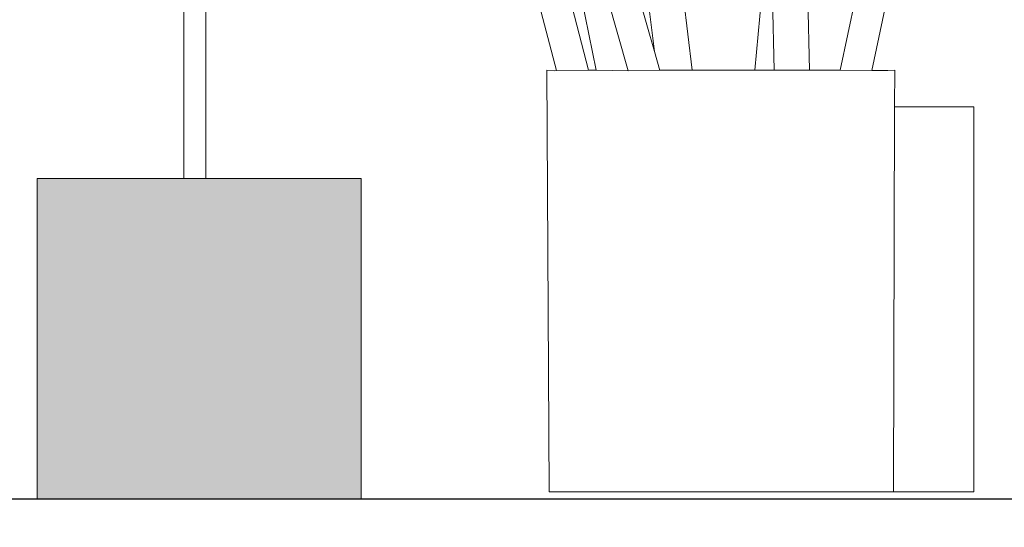
# Model space of a CAD drawing. Units: millimetres. Extents: x 7894 to 8038, y 6851 to 6951.
# Tile 32 of 49: x 7962.874 to 7968.188, y 6922.974 to 6925.713. Entities that reach past the tile are written whole.
import ezdxf

# ---------------------------------------------------------------- set-up
doc = ezdxf.new("R2010")
doc.units = ezdxf.units.MM
for name, color, linetype, lineweight in [('A-ANNO-DIMS', 2, 'Continuous', 18), ('A-FURN-ACCS', 8, 'Continuous', 13), ('A-FURN-SHLF', 7, 'Continuous', 30)]:
    doc.layers.add(name, color=color, linetype=linetype, lineweight=lineweight)
doc.layers.add('A-FURN-ACCS-PATT', color=116, linetype='Continuous', lineweight=9, true_color=0x136734)
doc.styles.get("Standard").update_dxf_attribs({"font": 'arial.ttf'})
doc.dimstyles.new('ISO-25', dxfattribs={"dimtxt": 1, "dimasz": 1, "dimexe": 1.25, "dimexo": 0.625, "dimtad": 1, "dimdec": 0, "dimlunit": 4, "dimtxsty": 'Standard', "dimcen": 2.5, "dimclrt": 1, "dimadec": 0, "dimazin": 0, "dimtfac": 1, "dimtdec": 0, "dimtmove": 0, "dimatfit": 3, "dimfxl": 1, "dimarcsym": 0})

# ---------------------------------------------------------------- blocks, each defined once
blk = doc.blocks.new('DISPLAY-LEAF-FINIAL-Z2_152')
for p, q in [((0.7416, 0, 2.1518), (0.7416, 1.0372, 2.1518)), ((0.8605, 0, 2.1518), (0.8605, 0.9923, 2.1518))]:
    blk.add_line(p, q)
blk = doc.blocks.new('DISPLAY-REED-SPRAY')
for p, q in [((0.5154, 1.5733), (0.4354, 1.9715)), ((1.5483, 0.9938), (1.529, 1.9891)), ((1.7657, 1.0095), (1.7415, 1.9798)), ((0.2181, 1.9336), (0.4198, 0.9626)), ((1.7698, 0.9258), (1.8607, 1.8783)), ((1.0617, 0.8114), (0.9453, 1.7069)), ((0.8459, 0.7666), (0.7293, 1.6887)), ((0.5782, 0.0032), (0.1619, 1.6106)), ((1.9375, 0.0029), (2.2747, 1.6026)), ((0, 1.5725), (0.4056, 0.0011)), ((0.9346, 0.1034), (0.5185, 1.5674)), ((2.1079, 0.0011), (2.44, 1.5729)), ((0.7924, 0), (0.3606, 1.5186)), ((0.6196, 0.0033), (0.4281, 0.9603)), ((1.5597, 0.991), (1.5609, 0.9349)), ((1.753, 0.8924), (1.7508, 0.9993)), ((1.4766, 0.0028), (1.5603, 0.9272)), ((1.5603, 0.9272), (1.5609, 0.9349)), ((1.5603, 0.9272), (1.5804, 0.0032)), ((1.753, 0.8924), (1.7551, 0.9145)), ((1.7713, 0.0032), (1.753, 0.8924)), ((1.1386, 0.003), (1.042, 0.8085)), ((0.9346, 0.1034), (0.8517, 0.7803)), ((0.9634, 0.002), (0.9346, 0.1034))]:
    blk.add_line(p, q)
blk = doc.blocks.new('*D23')
at = {"layer": 'A-ANNO-DIMS', "color": 0, "lineweight": -2, "transparency": 16777216}
for p, q in [((7940.0888, 6907.098), (7940.0888, 6947.7928)), ((7971.9356, 6928.989), (7971.9356, 6947.7928)), ((7941.0888, 6946.5428), (7970.9356, 6946.5428))]:
    blk.add_line(p, q, dxfattribs=at)
at = {"layer": 'A-ANNO-DIMS', "color": 0, "transparency": 16777216}
for points in [[(7941.0888, 6946.7095), (7941.0888, 6946.3762), (7940.0888, 6946.5428)], [(7970.9356, 6946.7095), (7970.9356, 6946.3762), (7971.9356, 6946.5428)]]:
    blk.add_solid(points, dxfattribs=at)
at = {"layer": 'Defpoints', "color": 0, "transparency": 16777216}
for p in [(7971.9356, 6946.5428), (7971.9356, 6928.364), (7940.0888, 6906.473)]:
    blk.add_point(p, dxfattribs=at)
at = {"layer": 'A-ANNO-DIMS', "color": 1, "transparency": 16777216, "insert": (7956.0122, 6947.6784), "char_height": 1, "attachment_point": 5}
blk.add_mtext('2\'-8"', dxfattribs=at)
blk = doc.blocks.new('*D28')
at = {"layer": 'A-ANNO-DIMS', "color": 0, "lineweight": -2, "transparency": 16777216}
for p, q in [((7960.8854, 6936.8804), (7975.2272, 6936.8804)), ((7973.9772, 6935.8804), (7973.9772, 6923.6283)), ((7971.8421, 6922.6283), (7975.2272, 6922.6283))]:
    blk.add_line(p, q, dxfattribs=at)
at = {"layer": 'A-ANNO-DIMS', "color": 0, "transparency": 16777216}
for points in [[(7973.8105, 6935.8804), (7974.1439, 6935.8804), (7973.9772, 6936.8804)], [(7973.8105, 6923.6283), (7974.1439, 6923.6283), (7973.9772, 6922.6283)]]:
    blk.add_solid(points, dxfattribs=at)
at = {"layer": 'Defpoints', "color": 0, "transparency": 16777216}
for p in [(7960.2604, 6936.8804), (7971.2171, 6922.6283), (7973.9772, 6922.6283)]:
    blk.add_point(p, dxfattribs=at)
at = {"layer": 'A-ANNO-DIMS', "color": 1, "transparency": 16777216, "insert": (7972.8351, 6929.7543), "char_height": 1, "attachment_point": 5, "rotation": 90}
blk.add_mtext('1\'-2 1/2"', dxfattribs=at)
blk = doc.blocks.new('*D31')
at = {"layer": 'A-ANNO-DIMS', "color": 0, "lineweight": -2, "transparency": 16777216}
for p, q in [((7973.9772, 6921.7198), (7973.9772, 6926.628)), ((7949.8107, 6920.7198), (7975.2272, 6920.7198)), ((7973.9772, 6918.7198), (7973.9772, 6920.7198)), ((7950.9654, 6918.7198), (7975.2272, 6918.7198)), ((7973.9772, 6917.7198), (7973.9772, 6916.7198))]:
    blk.add_line(p, q, dxfattribs=at)
at = {"layer": 'A-ANNO-DIMS', "color": 0, "transparency": 16777216}
for points in [[(7973.8105, 6921.7198), (7974.1439, 6921.7198), (7973.9772, 6920.7198)], [(7973.8105, 6917.7198), (7974.1439, 6917.7198), (7973.9772, 6918.7198)]]:
    blk.add_solid(points, dxfattribs=at)
at = {"layer": 'Defpoints', "color": 0, "transparency": 16777216}
for p in [(7949.1857, 6920.7198), (7973.9772, 6920.7198), (7950.3404, 6918.7198)]:
    blk.add_point(p, dxfattribs=at)
at = {"layer": 'A-ANNO-DIMS', "color": 1, "transparency": 16777216, "insert": (7972.8416, 6924.6739), "char_height": 1, "attachment_point": 5, "rotation": 90}
blk.add_mtext('0\'-2"', dxfattribs=at)

msp = doc.modelspace()

# ---------------------------------------------------------------- hatches: boundary and pattern name
at = {"layer": 'A-FURN-ACCS-PATT'}
h = msp.add_hatch(color=256, dxfattribs=at)
h.dxf.hatch_style = 1
h.paths.add_polyline_path([(7947.5161, 6931.8853), (7946.6774, 6931.8853), (7946.5585, 6931.8853), (7945.7683, 6931.8853), (7945.7683, 6930.1581), (7947.5161, 6930.1581)])
h.paths.add_polyline_path([(7947.4851, 6922.447), (7946.6464, 6922.447), (7946.5276, 6922.447), (7945.7373, 6922.447), (7945.7373, 6920.7198), (7947.4851, 6920.7198)])
h.paths.add_polyline_path([(7968.0212, 6935.881), (7967.1825, 6935.881), (7967.0637, 6935.881), (7966.2734, 6935.881), (7966.2734, 6934.1538), (7968.0212, 6934.1538)])
h.paths.add_polyline_path([(7960.6099, 6924.8555), (7959.7712, 6924.8555), (7959.6523, 6924.8555), (7958.862, 6924.8555), (7958.862, 6923.1283), (7960.6099, 6923.1283)])
h.paths.add_polyline_path([(7964.717, 6924.8555), (7963.8783, 6924.8555), (7963.7594, 6924.8555), (7962.9691, 6924.8555), (7962.9691, 6923.1283), (7964.717, 6923.1283)])
h.paths.add_polyline_path([(7971.0698, 6924.8555), (7970.2311, 6924.8555), (7970.1123, 6924.8555), (7969.322, 6924.8555), (7969.322, 6923.1283), (7971.0698, 6923.1283)])
h.paths.add_polyline_path([(7958.5294, 6908.7006), (7957.6907, 6908.7006), (7957.5718, 6908.7006), (7956.7815, 6908.7006), (7956.7815, 6906.9734), (7958.5294, 6906.9734)])

# ---------------------------------------------------------------- linework, layer by layer
at = {"layer": 'A-FURN-ACCS'}
for p, q in [((7965.7307, 6923.1653), (7965.7185, 6925.4412)), ((7965.7185, 6925.4412), (7965.7602, 6925.4381)), ((7965.7707, 6925.4388), (7965.7602, 6925.4381)), ((7965.9432, 6925.441), (7965.7707, 6925.4388)), ((7965.9846, 6925.441), (7965.9432, 6925.441)), ((7966.1575, 6925.4377), (7965.9846, 6925.441)), ((7966.3281, 6925.4407), (7966.1575, 6925.4377)), ((7966.5036, 6925.4407), (7966.3281, 6925.4407)), ((7966.8416, 6925.4405), (7966.5036, 6925.4407)), ((7966.9455, 6925.4409), (7966.8416, 6925.4405)), ((7967.1364, 6925.4409), (7966.9455, 6925.4409)), ((7967.3026, 6925.4406), (7967.1364, 6925.4409)), ((7967.473, 6925.4388), (7967.3026, 6925.4406)), ((7967.5587, 6925.4384), (7967.473, 6925.4388)), ((7967.5966, 6925.4412), (7967.5587, 6925.4384)), ((7967.596, 6925.2426), (7967.5966, 6925.4412)), ((7967.5895, 6923.1652), (7967.596, 6925.2426)), ((7967.596, 6925.2426), (7968.0225, 6925.2427)), ((7968.0225, 6925.2427), (7968.0225, 6923.1652)), ((7962.9691, 6923.1283, 2.1518), (7962.9691, 6924.8555, 2.1518)), ((7962.9691, 6924.8555, 2.1518), (7963.7594, 6924.8555, 2.1518)), ((7963.8783, 6924.8555, 2.1518), (7963.7594, 6924.8555, 2.1518)), ((7963.8783, 6924.8555, 2.1518), (7964.717, 6924.8555, 2.1518)), ((7964.717, 6923.1283, 2.1518), (7964.717, 6924.8555, 2.1518)), ((7965.8042, 6923.1652), (7965.7307, 6923.1653)), ((7965.8042, 6923.1652), (7965.9022, 6923.1652)), ((7965.9022, 6923.1652), (7965.9031, 6923.1652)), ((7967.5895, 6923.1652), (7965.9031, 6923.1652)), ((7968.0225, 6923.1652), (7967.5895, 6923.1652))]:
    msp.add_line(p, q, dxfattribs=at)
at = {"layer": 'A-FURN-SHLF'}
msp.add_line((7953.9136, 6923.1283, -7), (7971.2171, 6923.1283, -7), dxfattribs=at)

# ---------------------------------------------------------------- block references
at = {"layer": 'A-FURN-ACCS'}
for name, p in [('DISPLAY-LEAF-FINIAL-Z2_152', (7963.0178, 6924.8555)), ('DISPLAY-REED-SPRAY', (7965.365, 6925.4377))]:
    msp.add_blockref(name, p, dxfattribs=at)

# ---------------------------------------------------------------- dimensions: what is measured, and where the dimension line sits
at = {"layer": 'A-ANNO-DIMS'}
dim = msp.add_linear_dim(base=(7971.9356, 6946.5428), p1=(7940.0888, 6906.473), p2=(7971.9356, 6928.364), dimstyle='ISO-25', override={"dimdec": 1, "dimlfac": 1, "dimrnd": 0, "dimzin": 1, "dimdsep": 46, "dimlunit": 4, "dimfrac": 2}, dxfattribs=at)
dim.commit()
dim.dimension.update_dxf_attribs({"geometry": '*D23', "text_midpoint": (7956.0122, 6947.6784)})
for base, p1, p2, picture, middle in [((7973.9772, 6922.6283), (7960.2604, 6936.8804), (7971.2171, 6922.6283), '*D28', (7972.8351, 6929.7543)), ((7973.9772, 6920.7198), (7950.3404, 6918.7198), (7949.1857, 6920.7198), '*D31', (7972.8416, 6924.6739))]:
    dim = msp.add_linear_dim(base=base, p1=p1, p2=p2, angle=90, dimstyle='ISO-25', override={"dimdec": 1, "dimlfac": 1, "dimrnd": 0, "dimzin": 1, "dimdsep": 46, "dimlunit": 4, "dimfrac": 2}, dxfattribs=at)
    dim.commit()
    dim.dimension.update_dxf_attribs({"geometry": picture, "text_midpoint": middle})

doc.saveas('drawing.dxf')
